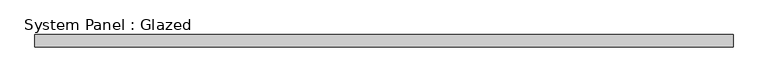
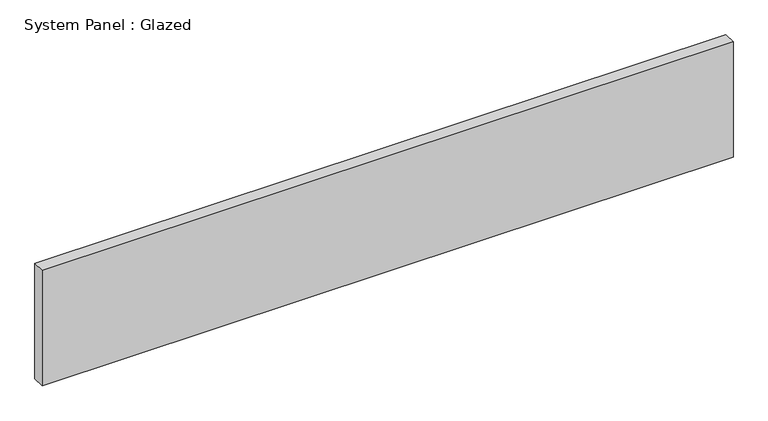
"""IFC4 building model written with IfcOpenShell, lengths in millimetres: plate geometry, System Panel : Glazed."""

from ifc_helpers import new_model, si_unit, origin, origin_with_axes, place, context, project, spatial, polyline, outline, extrude, source, transform, mapped, element, save


def system_panel_glazed_cac74210(model_context):
    return source(origin(), model_context, "Body", "SweptSolid", [
        extrude(outline(polyline([(711.2, 19.05), (-711.2, 19.05), (-711.2, 44.45), (711.2, 44.45), (711.2, 19.05)])), origin_with_axes(), (0.0, 0.0, 1.0), 251.1186703),
    ])


if __name__ == "__main__":
    model = new_model("IFC4")
    model_context = context("Model", 3, world=origin())
    ifc_project = project(units=[si_unit("LENGTHUNIT", "METRE", prefix="MILLI")], contexts=[model_context])
    site = spatial("IfcSite", under=ifc_project)
    building = spatial("IfcBuilding", under=site)
    placement = place(None, origin())
    system_panel_glazed_shape = system_panel_glazed_cac74210(model_context)
    element("IfcPlate", 1, ObjectType="System Panel : Glazed", at=placement, inside=building, context=model_context, shape_type="MappedRepresentation", body=[
        mapped(system_panel_glazed_shape, transform((0.0, 0.0, 0.0), x_axis=(1.0, 0.0, 0.0), y_axis=(0.0, 1.0, 0.0), z_axis=(0.0, 0.0, 1.0))),
    ])
    save(model, "model.ifc")

# Revit data of these elements
# Type "System Panel : Glazed"
#   Construction Type Id = "GSP4R"
#   Analytic Construction = "1/8 in Pilkington single glazing"
#   Visual Light Transmittance = 0.9
#   Solar Heat Gain Coefficient = 0.86
#   Heat Transfer Coefficient (U) = 1.18115 BTU/(h·ft²·°F)
#   Define Thermal Properties by = 1
# Element 1 (IfcPlate, "System Panel : Glazed")
#   Materials on its faces: "Glass"
# Materials
#   "Glass": class "Glass", colour RGB 0 128 192, transparency 0.75, Description = "Soda Lime Glass", Cost = 0
